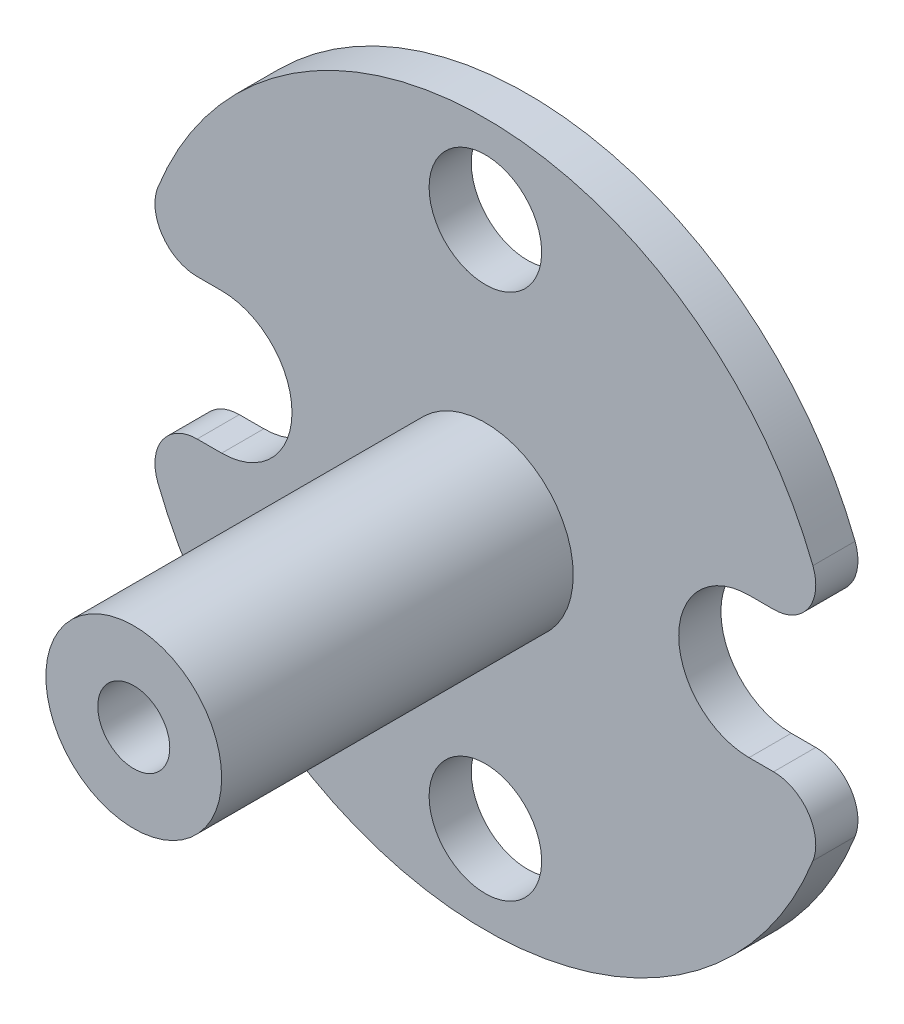
from build123d import *

# Parameters (mm, degrees)
PLATE_PROFILE_SKETCH_R    = 4.065
BASE_PLATE_0_12IN_DEPTH   = 3.048
PLATE_EDGE_FILLET_R0_12_R = 3.048
HUB_SKETCH_0_5_R          = 6.35
HUB_0_5_X_1IN_DEPTH       = 25.4


with BuildPart() as part:
    # Plate Profile Sketch → Base Plate 0.12in (new body)
    with BuildSketch(Plane.XY):
        with BuildLine():
            Line((-19.05, 5.08), (-24.886815787, 5.08))
            ThreePointArc((-24.886815787, 5.08), (0, 25.4), (24.886815787, 5.08))
            Line((24.886815787, 5.08), (19.05, 5.08))
            ThreePointArc((19.05, 5.08), (13.97, 0), (19.05, -5.08))
            Line((19.05, -5.08), (24.886815787, -5.08))
            ThreePointArc((24.886815787, -5.08), (0, -25.4), (-24.886815787, -5.08))
            Line((-24.886815787, -5.08), (-19.05, -5.08))
            ThreePointArc((-19.05, -5.08), (-13.97, 0), (-19.05, 5.08))
        make_face()
        with Locations(Location((0, 19.05, 0), (0, 0, 180))):
            Circle(PLATE_PROFILE_SKETCH_R, mode=Mode.SUBTRACT)
        with Locations(Location((0, -19.05, 0), (0, 0, 180))):
            Circle(PLATE_PROFILE_SKETCH_R, mode=Mode.SUBTRACT)
    extrude(amount=BASE_PLATE_0_12IN_DEPTH)

    # Plate Edge Fillet R0.12
    plate_edge_fillet_r0_12_edges = [part.edges().sort_by_distance(p)[0] for p in [
        (-24.886815787, 5.08, 1.524),
        (24.886815787, 5.08, 1.524),
        (24.886815787, -5.08, 1.524),
        (-24.886815787, -5.08, 1.524),
    ]]
    fillet(plate_edge_fillet_r0_12_edges, radius=PLATE_EDGE_FILLET_R0_12_R)

    # Hub Sketch Ø0.5 → Hub Ø0.5 x 1in (add)
    with BuildSketch(Plane.XY.offset(3.048)):
        Circle(HUB_SKETCH_0_5_R)
    extrude(amount=HUB_0_5_X_1IN_DEPTH)

    # Sketch5 → Hub Tapped Hole #10-24 (revolve, cut)
    with BuildSketch(Plane(origin=(0, 0, 28.448), x_dir=(0, -1, 0), z_dir=(1, 0, 0))):
        Polygon((0, 0), (0, 26.472108517), (2.45, 25), (2.45, 23), (2.6, 23), (2.6, 0), align=None)
    revolve(axis=Axis((0, 0, 34.798), (0, 0, -1)), mode=Mode.SUBTRACT)


solid = part.part
